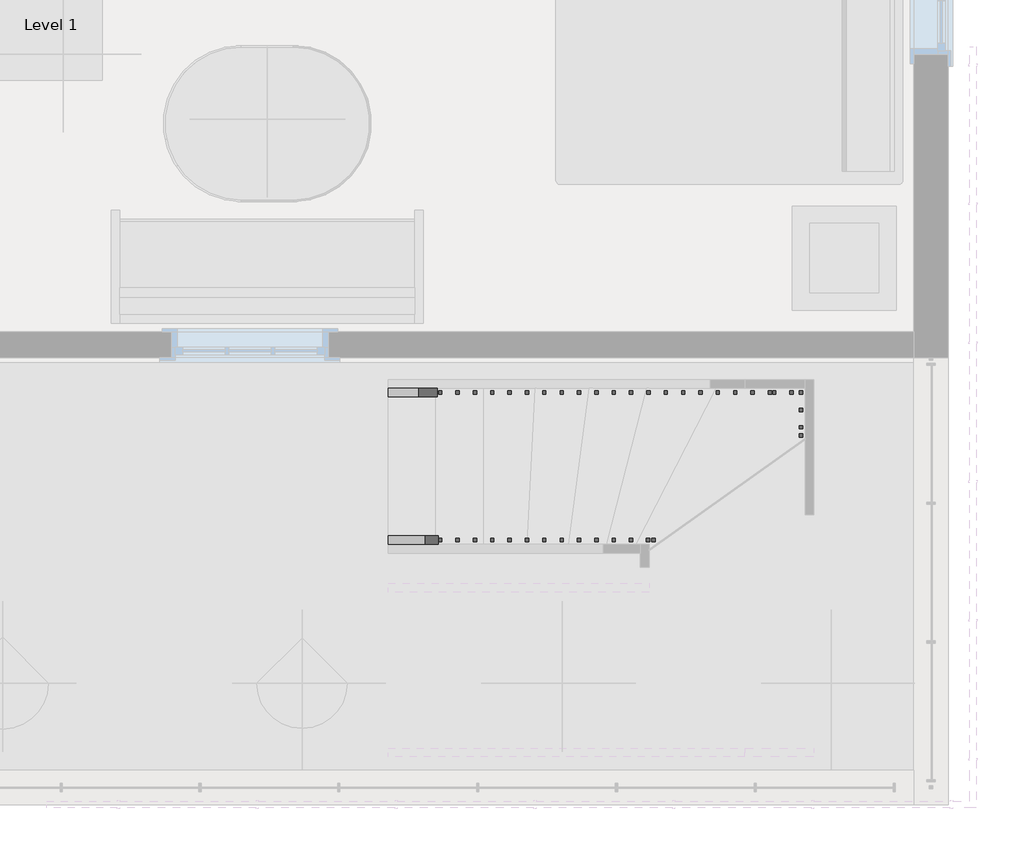
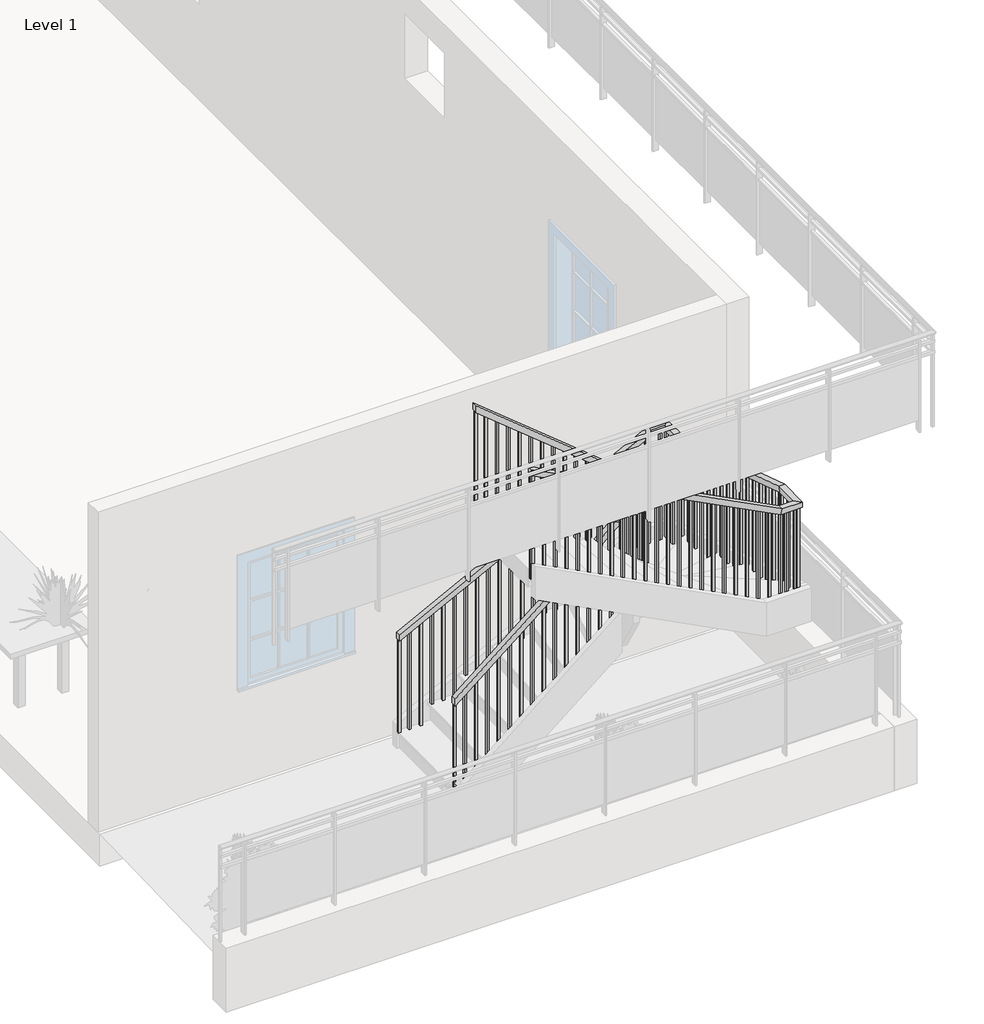
# One storey, part 2 of 5: 2 railings.
"""IFC4 building model written with IfcOpenShell, lengths in millimetres."""

from ifc_helpers import new_model, si_unit, frame, origin, place, context, project, spatial, polyline, outline, extrude, faceted_brep, element, save

model = new_model("IFC4")

# Units and contexts
model_context = context("Model", 3, world=origin())
ifc_project = project(units=[si_unit("LENGTHUNIT", "METRE", prefix="MILLI")], contexts=[model_context])

# Site, building, storey
site = spatial("IfcSite", under=ifc_project)
building = spatial("IfcBuilding", under=site)
storey = spatial("IfcBuildingStorey", under=building, Name="Level 1", Elevation=0.0)

# Railings
placement = place(None, origin())
element("IfcRailing", 1, ObjectType="Handrail - Rectangular", at=placement, inside=storey, context=model_context, shape_type="SolidModel", body=[
    faceted_brep([(-3203.9558053, -1061.3366944, 1025.2529681), (-3203.9558053, -1061.3366944, 959.7067088), (-3203.9558053, -1112.1366944, 959.7067088), (-3203.9558053, -1112.1366944, 1025.2529681), (-1752.4241134, -1061.3366944, 2208.7848338), (-1701.6241134, -1061.3366944, 2184.659247), (-1701.6241134, -1112.1366944, 2184.659247), (-1752.4241134, -1112.1366944, 2208.7848338), (-1752.4241134, -1061.3366944, 2414.6281882), (-1701.6241134, -1061.3366944, 2363.8281882), (-1701.6241134, -1112.1366944, 2363.8281882), (-1752.4241134, -1112.1366944, 2414.6281882), (-1625.4241134, -1061.3366944, 2414.6281882), (-1625.4241134, -1061.3366944, 2363.8281882), (-1676.2241134, -1112.1366944, 2363.8281882), (-1676.2241134, -1112.1366944, 2414.6281882), (-1625.4241134, -1188.3366944, 2414.6281882), (-1625.4241134, -1217.4580282, 2363.8281882), (-1676.2241134, -1217.4580282, 2363.8281882), (-1676.2241134, -1188.3366944, 2414.6281882), (-1625.4241134, -1315.3366944, 2631.5051451), (-1625.4241134, -1366.1366944, 2617.7256424), (-1676.2241134, -1366.1366944, 2617.7256424), (-1676.2241134, -1315.3366944, 2631.5051451), (-1625.4241134, -1315.3366944, 2837.3484995), (-1625.4241134, -1366.1366944, 2786.5484995), (-1676.2241134, -1366.1366944, 2786.5484995), (-1676.2241134, -1315.3366944, 2837.3484995), (-1625.4241134, -1442.3366944, 2837.3484995), (-1625.4241134, -1442.3366944, 2786.5484995), (-1676.2241134, -1391.5366944, 2786.5484995), (-1676.2241134, -1391.5366944, 2837.3484995), (-1752.4241134, -1442.3366944, 2837.3484995), (-1770.5095265, -1442.3366944, 2786.5484995), (-1770.5095265, -1391.5366944, 2786.5484995), (-1752.4241134, -1391.5366944, 2837.3484995), (-3203.9558053, -1442.3366944, 4020.8803652), (-3203.9558053, -1391.5366944, 4020.8803652), (-3203.9558053, -1391.5366944, 3955.3341059), (-3203.9558053, -1442.3366944, 3955.3341059)], [[[0, 1, 2, 3]], [[1, 0, 4, 5]], [[2, 1, 5, 6]], [[3, 2, 6, 7]], [[0, 3, 7, 4]], [[5, 4, 8, 9]], [[6, 5, 9, 10]], [[7, 6, 10, 11]], [[4, 7, 11, 8]], [[9, 8, 12, 13]], [[10, 9, 13, 14]], [[11, 10, 14, 15]], [[8, 11, 15, 12]], [[13, 12, 16, 17]], [[14, 13, 17, 18]], [[15, 14, 18, 19]], [[12, 15, 19, 16]], [[17, 16, 20, 21]], [[18, 17, 21, 22]], [[19, 18, 22, 23]], [[16, 19, 23, 20]], [[21, 20, 24, 25]], [[22, 21, 25, 26]], [[23, 22, 26, 27]], [[20, 23, 27, 24]], [[25, 24, 28, 29]], [[26, 25, 29, 30]], [[27, 26, 30, 31]], [[24, 27, 31, 28]], [[29, 28, 32, 33]], [[30, 29, 33, 34]], [[31, 30, 34, 35]], [[28, 31, 35, 32]], [[36, 37, 38, 39]], [[33, 32, 36, 39]], [[34, 33, 39, 38]], [[35, 34, 38, 37]], [[32, 35, 37, 36]]]),
    extrude(outline(polyline([(3866.2231262, -3094.6664698), (3881.7558784, -3113.7164698), (2878.6666667, -3113.7164698), (2878.6666667, -3094.6664698), (3866.2231262, -3094.6664698)])), frame((0.0, -1426.4616944, 0.0), z_axis=(0.0, 1.0, 0.0), x_axis=(0.0, 0.0, 1.0)), (0.0, 0.0, 1.0), 19.05),
    extrude(outline(polyline([(3783.3817813, -2993.0664698), (3798.9145334, -3012.1164698), (2878.6666667, -3012.1164698), (2878.6666667, -2993.0664698), (3783.3817813, -2993.0664698)])), frame((0.0, -1426.4616944, 0.0), z_axis=(0.0, 1.0, 0.0), x_axis=(0.0, 0.0, 1.0)), (0.0, 0.0, 1.0), 19.05),
    extrude(outline(polyline([(3700.5404364, -2891.4664698), (3716.0731885, -2910.5164698), (2709.3333333, -2910.5164698), (2709.3333333, -2891.4664698), (3700.5404364, -2891.4664698)])), frame((0.0, -1426.4616944, 0.0), z_axis=(0.0, 1.0, 0.0), x_axis=(0.0, 0.0, 1.0)), (0.0, 0.0, 1.0), 19.05),
    extrude(outline(polyline([(3617.6990914, -2789.8664698), (3633.2318436, -2808.9164698), (2709.3333333, -2808.9164698), (2709.3333333, -2789.8664698), (3617.6990914, -2789.8664698)])), frame((0.0, -1426.4616944, 0.0), z_axis=(0.0, 1.0, 0.0), x_axis=(0.0, 0.0, 1.0)), (0.0, 0.0, 1.0), 19.05),
    extrude(outline(polyline([(3534.8577465, -2688.2664698), (3550.3904987, -2707.3164698), (2709.3333333, -2707.3164698), (2709.3333333, -2688.2664698), (3534.8577465, -2688.2664698)])), frame((0.0, -1426.4616944, 0.0), z_axis=(0.0, 1.0, 0.0), x_axis=(0.0, 0.0, 1.0)), (0.0, 0.0, 1.0), 19.05),
    extrude(outline(polyline([(3452.0164016, -2586.6664698), (3467.5491538, -2605.7164698), (2540.0, -2605.7164698), (2540.0, -2586.6664698), (3452.0164016, -2586.6664698)])), frame((0.0, -1426.4616944, 0.0), z_axis=(0.0, 1.0, 0.0), x_axis=(0.0, 0.0, 1.0)), (0.0, 0.0, 1.0), 19.05),
    extrude(outline(polyline([(3369.1750567, -2485.0664698), (3384.7078088, -2504.1164698), (2540.0, -2504.1164698), (2540.0, -2485.0664698), (3369.1750567, -2485.0664698)])), frame((0.0, -1426.4616944, 0.0), z_axis=(0.0, 1.0, 0.0), x_axis=(0.0, 0.0, 1.0)), (0.0, 0.0, 1.0), 19.05),
    extrude(outline(polyline([(3286.3337117, -2383.4664698), (3301.8664639, -2402.5164698), (2540.0, -2402.5164698), (2540.0, -2383.4664698), (3286.3337117, -2383.4664698)])), frame((0.0, -1426.4616944, 0.0), z_axis=(0.0, 1.0, 0.0), x_axis=(0.0, 0.0, 1.0)), (0.0, 0.0, 1.0), 19.05),
    extrude(outline(polyline([(3203.4923668, -2281.8664698), (3219.025119, -2300.9164698), (2370.6666667, -2300.9164698), (2370.6666667, -2281.8664698), (3203.4923668, -2281.8664698)])), frame((0.0, -1426.4616944, 0.0), z_axis=(0.0, 1.0, 0.0), x_axis=(0.0, 0.0, 1.0)), (0.0, 0.0, 1.0), 19.05),
    extrude(outline(polyline([(3120.6510219, -2180.2664698), (3136.1837741, -2199.3164698), (2370.6666667, -2199.3164698), (2370.6666667, -2180.2664698), (3120.6510219, -2180.2664698)])), frame((0.0, -1426.4616944, 0.0), z_axis=(0.0, 1.0, 0.0), x_axis=(0.0, 0.0, 1.0)), (0.0, 0.0, 1.0), 19.05),
    extrude(outline(polyline([(3037.809677, -2078.6664698), (3053.3424291, -2097.7164698), (2201.3333333, -2097.7164698), (2201.3333333, -2078.6664698), (3037.809677, -2078.6664698)])), frame((0.0, -1426.4616944, 0.0), z_axis=(0.0, 1.0, 0.0), x_axis=(0.0, 0.0, 1.0)), (0.0, 0.0, 1.0), 19.05),
    extrude(outline(polyline([(2954.9683321, -1977.0664698), (2970.5010842, -1996.1164698), (2201.3333333, -1996.1164698), (2201.3333333, -1977.0664698), (2954.9683321, -1977.0664698)])), frame((0.0, -1426.4616944, 0.0), z_axis=(0.0, 1.0, 0.0), x_axis=(0.0, 0.0, 1.0)), (0.0, 0.0, 1.0), 19.05),
    extrude(outline(polyline([(2872.1269871, -1875.4664698), (2887.6597393, -1894.5164698), (2032.0, -1894.5164698), (2032.0, -1875.4664698), (2872.1269871, -1875.4664698)])), frame((0.0, -1426.4616944, 0.0), z_axis=(0.0, 1.0, 0.0), x_axis=(0.0, 0.0, 1.0)), (0.0, 0.0, 1.0), 19.05),
    extrude(outline(polyline([(2789.2856422, -1773.8664698), (2804.8183944, -1792.9164698), (2032.0, -1792.9164698), (2032.0, -1773.8664698), (2789.2856422, -1773.8664698)])), frame((0.0, -1426.4616944, 0.0), z_axis=(0.0, 1.0, 0.0), x_axis=(0.0, 0.0, 1.0)), (0.0, 0.0, 1.0), 19.05),
    extrude(outline(polyline([(-1314.2475981, 2529.115018), (-1295.1975981, 2496.5834745), (-1295.1975981, 1524.0), (-1314.2475981, 1524.0), (-1314.2475981, 2529.115018)])), frame((-1660.3491134, 0.0, 0.0), z_axis=(1.0, 0.0, 0.0), x_axis=(0.0, 1.0, 0.0)), (0.0, 0.0, 1.0), 19.05),
    extrude(outline(polyline([(-1212.6475981, 2355.6134525), (-1193.5975981, 2323.0819089), (-1193.5975981, 1524.0), (-1212.6475981, 1524.0), (-1212.6475981, 2355.6134525)])), frame((-1660.3491134, 0.0, 0.0), z_axis=(1.0, 0.0, 0.0), x_axis=(0.0, 1.0, 0.0)), (0.0, 0.0, 1.0), 19.05),
    extrude(outline(polyline([(2127.2519138, -1772.0308053), (2111.7191617, -1791.0808053), (1016.0, -1791.0808053), (1016.0, -1772.0308053), (2127.2519138, -1772.0308053)])), frame((0.0, -1096.2616944, 0.0), z_axis=(0.0, 1.0, 0.0), x_axis=(0.0, 0.0, 1.0)), (0.0, 0.0, 1.0), 19.05),
    extrude(outline(polyline([(2044.4105689, -1873.6308053), (2028.8778167, -1892.6808053), (1016.0, -1892.6808053), (1016.0, -1873.6308053), (2044.4105689, -1873.6308053)])), frame((0.0, -1096.2616944, 0.0), z_axis=(0.0, 1.0, 0.0), x_axis=(0.0, 0.0, 1.0)), (0.0, 0.0, 1.0), 19.05),
    extrude(outline(polyline([(1961.569224, -1975.2308053), (1946.0364718, -1994.2808053), (846.6666667, -1994.2808053), (846.6666667, -1975.2308053), (1961.569224, -1975.2308053)])), frame((0.0, -1096.2616944, 0.0), z_axis=(0.0, 1.0, 0.0), x_axis=(0.0, 0.0, 1.0)), (0.0, 0.0, 1.0), 19.05),
    extrude(outline(polyline([(1878.7278791, -2076.8308053), (1863.1951269, -2095.8808053), (846.6666667, -2095.8808053), (846.6666667, -2076.8308053), (1878.7278791, -2076.8308053)])), frame((0.0, -1096.2616944, 0.0), z_axis=(0.0, 1.0, 0.0), x_axis=(0.0, 0.0, 1.0)), (0.0, 0.0, 1.0), 19.05),
    extrude(outline(polyline([(1795.8865341, -2178.4308053), (1780.353782, -2197.4808053), (677.3333333, -2197.4808053), (677.3333333, -2178.4308053), (1795.8865341, -2178.4308053)])), frame((0.0, -1096.2616944, 0.0), z_axis=(0.0, 1.0, 0.0), x_axis=(0.0, 0.0, 1.0)), (0.0, 0.0, 1.0), 19.05),
    extrude(outline(polyline([(1713.0451892, -2280.0308053), (1697.5124371, -2299.0808053), (677.3333333, -2299.0808053), (677.3333333, -2280.0308053), (1713.0451892, -2280.0308053)])), frame((0.0, -1096.2616944, 0.0), z_axis=(0.0, 1.0, 0.0), x_axis=(0.0, 0.0, 1.0)), (0.0, 0.0, 1.0), 19.05),
    extrude(outline(polyline([(1630.2038443, -2381.6308053), (1614.6710921, -2400.6808053), (508.0, -2400.6808053), (508.0, -2381.6308053), (1630.2038443, -2381.6308053)])), frame((0.0, -1096.2616944, 0.0), z_axis=(0.0, 1.0, 0.0), x_axis=(0.0, 0.0, 1.0)), (0.0, 0.0, 1.0), 19.05),
    extrude(outline(polyline([(1547.3624994, -2483.2308053), (1531.8297472, -2502.2808053), (508.0, -2502.2808053), (508.0, -2483.2308053), (1547.3624994, -2483.2308053)])), frame((0.0, -1096.2616944, 0.0), z_axis=(0.0, 1.0, 0.0), x_axis=(0.0, 0.0, 1.0)), (0.0, 0.0, 1.0), 19.05),
    extrude(outline(polyline([(1464.5211545, -2584.8308053), (1448.9884023, -2603.8808053), (508.0, -2603.8808053), (508.0, -2584.8308053), (1464.5211545, -2584.8308053)])), frame((0.0, -1096.2616944, 0.0), z_axis=(0.0, 1.0, 0.0), x_axis=(0.0, 0.0, 1.0)), (0.0, 0.0, 1.0), 19.05),
    extrude(outline(polyline([(1381.6798095, -2686.4308053), (1366.1470574, -2705.4808053), (338.6666667, -2705.4808053), (338.6666667, -2686.4308053), (1381.6798095, -2686.4308053)])), frame((0.0, -1096.2616944, 0.0), z_axis=(0.0, 1.0, 0.0), x_axis=(0.0, 0.0, 1.0)), (0.0, 0.0, 1.0), 19.05),
    extrude(outline(polyline([(1298.8384646, -2788.0308053), (1283.3057124, -2807.0808053), (338.6666667, -2807.0808053), (338.6666667, -2788.0308053), (1298.8384646, -2788.0308053)])), frame((0.0, -1096.2616944, 0.0), z_axis=(0.0, 1.0, 0.0), x_axis=(0.0, 0.0, 1.0)), (0.0, 0.0, 1.0), 19.05),
    extrude(outline(polyline([(1215.9971197, -2889.6308053), (1200.4643675, -2908.6808053), (338.6666667, -2908.6808053), (338.6666667, -2889.6308053), (1215.9971197, -2889.6308053)])), frame((0.0, -1096.2616944, 0.0), z_axis=(0.0, 1.0, 0.0), x_axis=(0.0, 0.0, 1.0)), (0.0, 0.0, 1.0), 19.05),
    extrude(outline(polyline([(1133.1557748, -2991.2308053), (1117.6230226, -3010.2808053), (169.3333333, -3010.2808053), (169.3333333, -2991.2308053), (1133.1557748, -2991.2308053)])), frame((0.0, -1096.2616944, 0.0), z_axis=(0.0, 1.0, 0.0), x_axis=(0.0, 0.0, 1.0)), (0.0, 0.0, 1.0), 19.05),
    extrude(outline(polyline([(1050.3144298, -3092.8308053), (1034.7816777, -3111.8808053), (169.3333333, -3111.8808053), (169.3333333, -3092.8308053), (1050.3144298, -3092.8308053)])), frame((0.0, -1096.2616944, 0.0), z_axis=(0.0, 1.0, 0.0), x_axis=(0.0, 0.0, 1.0)), (0.0, 0.0, 1.0), 19.05),
    extrude(outline(polyline([(-1672.2664698, -1407.4116944), (-1672.2664698, -1426.4616944), (-1691.3164698, -1426.4616944), (-1691.3164698, -1407.4116944), (-1672.2664698, -1407.4116944)])), frame((0.0, 0.0, 1862.6666667), z_axis=(0.0, 0.0, 1.0), x_axis=(1.0, 0.0, 0.0)), (0.0, 0.0, 1.0), 923.8818329),
    extrude(outline(polyline([(-1660.3491134, -1407.4116944), (-1641.2991134, -1407.4116944), (-1641.2991134, -1426.4616944), (-1660.3491134, -1426.4616944), (-1660.3491134, -1407.4116944)])), frame((0.0, 0.0, 1862.6666667), z_axis=(0.0, 0.0, 1.0), x_axis=(1.0, 0.0, 0.0)), (0.0, 0.0, 1.0), 923.8818329),
    extrude(outline(polyline([(-1660.3491134, -1392.6257906), (-1641.2991134, -1392.6257906), (-1641.2991134, -1411.6757906), (-1660.3491134, -1411.6757906), (-1660.3491134, -1392.6257906)])), frame((0.0, 0.0, 1693.3333333), z_axis=(0.0, 0.0, 1.0), x_axis=(1.0, 0.0, 0.0)), (0.0, 0.0, 1.0), 1093.2151662),
    extrude(outline(polyline([(-1660.3491134, -1091.9975981), (-1641.2991134, -1091.9975981), (-1641.2991134, -1111.0475981), (-1660.3491134, -1111.0475981), (-1660.3491134, -1091.9975981)])), frame((0.0, 0.0, 1354.6666667), z_axis=(0.0, 0.0, 1.0), x_axis=(1.0, 0.0, 0.0)), (0.0, 0.0, 1.0), 1009.1615215),
    extrude(outline(polyline([(-1660.3491134, -1096.2616944), (-1660.3491134, -1077.2116944), (-1641.2991134, -1077.2116944), (-1641.2991134, -1096.2616944), (-1660.3491134, -1096.2616944)])), frame((0.0, 0.0, 1185.3333333), z_axis=(0.0, 0.0, 1.0), x_axis=(1.0, 0.0, 0.0)), (0.0, 0.0, 1.0), 1178.4948549),
    extrude(outline(polyline([(-1691.3164698, -1096.2616944), (-1691.3164698, -1077.2116944), (-1672.2664698, -1077.2116944), (-1672.2664698, -1096.2616944), (-1691.3164698, -1096.2616944)])), frame((0.0, 0.0, 1185.3333333), z_axis=(0.0, 0.0, 1.0), x_axis=(1.0, 0.0, 0.0)), (0.0, 0.0, 1.0), 1178.4948549),
    extrude(outline(polyline([(3939.8013537, -3184.9058053), (3955.3341059, -3203.9558053), (2878.6666667, -3203.9558053), (2878.6666667, -3184.9058053), (3939.8013537, -3184.9058053)])), frame((0.0, -1426.4616944, 0.0), z_axis=(0.0, 1.0, 0.0), x_axis=(0.0, 0.0, 1.0)), (0.0, 0.0, 1.0), 19.05),
    extrude(outline(polyline([(975.239461, -3184.9058053), (959.7067088, -3203.9558053), (169.3333333, -3203.9558053), (169.3333333, -3184.9058053), (975.239461, -3184.9058053)])), frame((0.0, -1096.2616944, 0.0), z_axis=(0.0, 1.0, 0.0), x_axis=(0.0, 0.0, 1.0)), (0.0, 0.0, 1.0), 19.05),
])
element("IfcRailing", 2, ObjectType="Handrail - Rectangular", at=placement, inside=storey, context=model_context, shape_type="SolidModel", body=[
    faceted_brep([(-3203.9558053, -197.7366944, 1109.0771751), (-3203.9558053, -197.7366944, 1051.9280057), (-3203.9558053, -248.5366944, 1051.9280057), (-3203.9558053, -248.5366944, 1109.0771751), (-943.9739488, -197.7366944, 2273.7644996), (-931.6538975, -197.7366944, 2222.9644996), (-931.6538975, -248.5366944, 2222.9644996), (-943.9739488, -248.5366944, 2273.7644996), (-761.8241134, -197.7366944, 2273.7644996), (-761.8241134, -197.7366944, 2222.9644996), (-812.6241134, -248.5366944, 2222.9644996), (-812.6241134, -248.5366944, 2273.7644996), (-761.8241134, -474.890647, 2273.7644996), (-761.8241134, -482.8412231, 2222.9644996), (-812.6241134, -482.8412231, 2222.9644996), (-812.6241134, -474.890647, 2273.7644996), (-761.8241134, -2028.7827418, 2772.3688337), (-761.8241134, -2036.7333179, 2721.5688337), (-812.6241134, -2036.7333179, 2721.5688337), (-812.6241134, -2028.7827418, 2772.3688337), (-761.8241134, -2305.9366944, 2772.3688337), (-761.8241134, -2305.9366944, 2721.5688337), (-812.6241134, -2255.1366944, 2721.5688337), (-812.6241134, -2255.1366944, 2772.3688337), (-943.9739488, -2305.9366944, 2772.3688337), (-956.2940001, -2305.9366944, 2721.5688337), (-956.2940001, -2255.1366944, 2721.5688337), (-943.9739488, -2255.1366944, 2772.3688337), (-3203.9558053, -2305.9366944, 3937.0561582), (-3203.9558053, -2255.1366944, 3937.0561582), (-3203.9558053, -2255.1366944, 3879.9069889), (-3203.9558053, -2305.9366944, 3879.9069889)], [[[0, 1, 2, 3]], [[1, 0, 4, 5]], [[2, 1, 5, 6]], [[3, 2, 6, 7]], [[0, 3, 7, 4]], [[5, 4, 8, 9]], [[6, 5, 9, 10]], [[7, 6, 10, 11]], [[4, 7, 11, 8]], [[9, 8, 12, 13]], [[10, 9, 13, 14]], [[11, 10, 14, 15]], [[8, 11, 15, 12]], [[13, 12, 16, 17]], [[14, 13, 17, 18]], [[15, 14, 18, 19]], [[12, 15, 19, 16]], [[17, 16, 20, 21]], [[18, 17, 21, 22]], [[19, 18, 22, 23]], [[16, 19, 23, 20]], [[21, 20, 24, 25]], [[22, 21, 25, 26]], [[23, 22, 26, 27]], [[20, 23, 27, 24]], [[28, 29, 30, 31]], [[25, 24, 28, 31]], [[26, 25, 31, 30]], [[27, 26, 30, 29]], [[24, 27, 29, 28]]]),
    extrude(outline(polyline([(3872.0443296, -3188.6989488), (2878.6666667, -3188.6989488), (2878.6666667, -3169.6489488), (3862.2268642, -3169.6489488), (3872.0443296, -3188.6989488)])), frame((0.0, -2290.0616944, 0.0), z_axis=(0.0, 1.0, 0.0), x_axis=(0.0, 0.0, 1.0)), (0.0, 0.0, 1.0), 19.05),
    extrude(outline(polyline([(3819.6845145, -3087.0989488), (2878.6666667, -3087.0989488), (2878.6666667, -3068.0489488), (3809.8670491, -3068.0489488), (3819.6845145, -3087.0989488)])), frame((0.0, -2290.0616944, 0.0), z_axis=(0.0, 1.0, 0.0), x_axis=(0.0, 0.0, 1.0)), (0.0, 0.0, 1.0), 19.05),
    extrude(outline(polyline([(3767.3246993, -2985.4989488), (2878.6666667, -2985.4989488), (2878.6666667, -2966.4489488), (3757.507234, -2966.4489488), (3767.3246993, -2985.4989488)])), frame((0.0, -2290.0616944, 0.0), z_axis=(0.0, 1.0, 0.0), x_axis=(0.0, 0.0, 1.0)), (0.0, 0.0, 1.0), 19.05),
    extrude(outline(polyline([(3714.9648842, -2883.8989488), (2709.3333333, -2883.8989488), (2709.3333333, -2864.8489488), (3705.1474189, -2864.8489488), (3714.9648842, -2883.8989488)])), frame((0.0, -2290.0616944, 0.0), z_axis=(0.0, 1.0, 0.0), x_axis=(0.0, 0.0, 1.0)), (0.0, 0.0, 1.0), 19.05),
    extrude(outline(polyline([(3662.6050691, -2782.2989488), (2709.3333333, -2782.2989488), (2709.3333333, -2763.2489488), (3652.7876038, -2763.2489488), (3662.6050691, -2782.2989488)])), frame((0.0, -2290.0616944, 0.0), z_axis=(0.0, 1.0, 0.0), x_axis=(0.0, 0.0, 1.0)), (0.0, 0.0, 1.0), 19.05),
    extrude(outline(polyline([(3610.245254, -2680.6989488), (2709.3333333, -2680.6989488), (2709.3333333, -2661.6489488), (3600.4277887, -2661.6489488), (3610.245254, -2680.6989488)])), frame((0.0, -2290.0616944, 0.0), z_axis=(0.0, 1.0, 0.0), x_axis=(0.0, 0.0, 1.0)), (0.0, 0.0, 1.0), 19.05),
    extrude(outline(polyline([(3557.8854389, -2579.0989488), (2540.0, -2579.0989488), (2540.0, -2560.0489488), (3548.0679735, -2560.0489488), (3557.8854389, -2579.0989488)])), frame((0.0, -2290.0616944, 0.0), z_axis=(0.0, 1.0, 0.0), x_axis=(0.0, 0.0, 1.0)), (0.0, 0.0, 1.0), 19.05),
    extrude(outline(polyline([(3505.5256238, -2477.4989488), (2540.0, -2477.4989488), (2540.0, -2458.4489488), (3495.7081584, -2458.4489488), (3505.5256238, -2477.4989488)])), frame((0.0, -2290.0616944, 0.0), z_axis=(0.0, 1.0, 0.0), x_axis=(0.0, 0.0, 1.0)), (0.0, 0.0, 1.0), 19.05),
    extrude(outline(polyline([(3453.1658086, -2375.8989488), (2540.0, -2375.8989488), (2540.0, -2356.8489488), (3443.3483433, -2356.8489488), (3453.1658086, -2375.8989488)])), frame((0.0, -2290.0616944, 0.0), z_axis=(0.0, 1.0, 0.0), x_axis=(0.0, 0.0, 1.0)), (0.0, 0.0, 1.0), 19.05),
    extrude(outline(polyline([(3400.8059935, -2274.2989488), (2370.6666667, -2274.2989488), (2370.6666667, -2255.2489488), (3390.9885282, -2255.2489488), (3400.8059935, -2274.2989488)])), frame((0.0, -2290.0616944, 0.0), z_axis=(0.0, 1.0, 0.0), x_axis=(0.0, 0.0, 1.0)), (0.0, 0.0, 1.0), 19.05),
    extrude(outline(polyline([(3348.4461784, -2172.6989488), (2370.6666667, -2172.6989488), (2370.6666667, -2153.6489488), (3338.6287131, -2153.6489488), (3348.4461784, -2172.6989488)])), frame((0.0, -2290.0616944, 0.0), z_axis=(0.0, 1.0, 0.0), x_axis=(0.0, 0.0, 1.0)), (0.0, 0.0, 1.0), 19.05),
    extrude(outline(polyline([(3296.0863633, -2071.0989488), (2370.6666667, -2071.0989488), (2370.6666667, -2052.0489488), (3286.268898, -2052.0489488), (3296.0863633, -2071.0989488)])), frame((0.0, -2290.0616944, 0.0), z_axis=(0.0, 1.0, 0.0), x_axis=(0.0, 0.0, 1.0)), (0.0, 0.0, 1.0), 19.05),
    extrude(outline(polyline([(3243.7265482, -1969.4989488), (2201.3333333, -1969.4989488), (2201.3333333, -1950.4489488), (3233.9090828, -1950.4489488), (3243.7265482, -1969.4989488)])), frame((0.0, -2290.0616944, 0.0), z_axis=(0.0, 1.0, 0.0), x_axis=(0.0, 0.0, 1.0)), (0.0, 0.0, 1.0), 19.05),
    extrude(outline(polyline([(3191.3667331, -1867.8989488), (2201.3333333, -1867.8989488), (2201.3333333, -1848.8489488), (3181.5492677, -1848.8489488), (3191.3667331, -1867.8989488)])), frame((0.0, -2290.0616944, 0.0), z_axis=(0.0, 1.0, 0.0), x_axis=(0.0, 0.0, 1.0)), (0.0, 0.0, 1.0), 19.05),
    extrude(outline(polyline([(3139.0069179, -1766.2989488), (2201.3333333, -1766.2989488), (2201.3333333, -1747.2489488), (3129.1894526, -1747.2489488), (3139.0069179, -1766.2989488)])), frame((0.0, -2290.0616944, 0.0), z_axis=(0.0, 1.0, 0.0), x_axis=(0.0, 0.0, 1.0)), (0.0, 0.0, 1.0), 19.05),
    extrude(outline(polyline([(3086.6471028, -1664.6989488), (2032.0, -1664.6989488), (2032.0, -1645.6489488), (3076.8296375, -1645.6489488), (3086.6471028, -1664.6989488)])), frame((0.0, -2290.0616944, 0.0), z_axis=(0.0, 1.0, 0.0), x_axis=(0.0, 0.0, 1.0)), (0.0, 0.0, 1.0), 19.05),
    extrude(outline(polyline([(3034.2872877, -1563.0989488), (2032.0, -1563.0989488), (2032.0, -1544.0489488), (3024.4698224, -1544.0489488), (3034.2872877, -1563.0989488)])), frame((0.0, -2290.0616944, 0.0), z_axis=(0.0, 1.0, 0.0), x_axis=(0.0, 0.0, 1.0)), (0.0, 0.0, 1.0), 19.05),
    extrude(outline(polyline([(2981.9274726, -1461.4989488), (2032.0, -1461.4989488), (2032.0, -1442.4489488), (2972.1100073, -1442.4489488), (2981.9274726, -1461.4989488)])), frame((0.0, -2290.0616944, 0.0), z_axis=(0.0, 1.0, 0.0), x_axis=(0.0, 0.0, 1.0)), (0.0, 0.0, 1.0), 19.05),
    extrude(outline(polyline([(2929.5676575, -1359.8989488), (2032.0, -1359.8989488), (2032.0, -1340.8489488), (2919.7501921, -1340.8489488), (2929.5676575, -1359.8989488)])), frame((0.0, -2290.0616944, 0.0), z_axis=(0.0, 1.0, 0.0), x_axis=(0.0, 0.0, 1.0)), (0.0, 0.0, 1.0), 19.05),
    extrude(outline(polyline([(2877.2078424, -1258.2989488), (1862.6666667, -1258.2989488), (1862.6666667, -1239.2489488), (2867.390377, -1239.2489488), (2877.2078424, -1258.2989488)])), frame((0.0, -2290.0616944, 0.0), z_axis=(0.0, 1.0, 0.0), x_axis=(0.0, 0.0, 1.0)), (0.0, 0.0, 1.0), 19.05),
    extrude(outline(polyline([(2824.8480272, -1156.6989488), (1862.6666667, -1156.6989488), (1862.6666667, -1137.6489488), (2815.0305619, -1137.6489488), (2824.8480272, -1156.6989488)])), frame((0.0, -2290.0616944, 0.0), z_axis=(0.0, 1.0, 0.0), x_axis=(0.0, 0.0, 1.0)), (0.0, 0.0, 1.0), 19.05),
    extrude(outline(polyline([(2772.4882121, -1055.0989488), (1862.6666667, -1055.0989488), (1862.6666667, -1036.0489488), (2762.6707468, -1036.0489488), (2772.4882121, -1055.0989488)])), frame((0.0, -2290.0616944, 0.0), z_axis=(0.0, 1.0, 0.0), x_axis=(0.0, 0.0, 1.0)), (0.0, 0.0, 1.0), 19.05),
    extrude(outline(polyline([(-879.2991134, -2290.0616944), (-898.3491134, -2290.0616944), (-898.3491134, -2271.0116944), (-879.2991134, -2271.0116944), (-879.2991134, -2290.0616944)])), frame((0.0, 0.0, 1862.6666667), z_axis=(0.0, 0.0, 1.0), x_axis=(1.0, 0.0, 0.0)), (0.0, 0.0, 1.0), 858.902167),
    extrude(outline(polyline([(-777.6991134, -2222.4577418), (-777.6991134, -2241.5077418), (-796.7491134, -2241.5077418), (-796.7491134, -2222.4577418), (-777.6991134, -2222.4577418)])), frame((0.0, 0.0, 1862.6666667), z_axis=(0.0, 0.0, 1.0), x_axis=(1.0, 0.0, 0.0)), (0.0, 0.0, 1.0), 858.902167),
    extrude(outline(polyline([(-777.6991134, -2120.8577418), (-777.6991134, -2139.9077418), (-796.7491134, -2139.9077418), (-796.7491134, -2120.8577418), (-777.6991134, -2120.8577418)])), frame((0.0, 0.0, 1862.6666667), z_axis=(0.0, 0.0, 1.0), x_axis=(1.0, 0.0, 0.0)), (0.0, 0.0, 1.0), 858.902167),
    extrude(outline(polyline([(-1989.365647, 2706.3697564), (-1989.365647, 1693.3333333), (-2008.415647, 1693.3333333), (-2008.415647, 2712.4824155), (-1989.365647, 2706.3697564)])), frame((-796.7491134, 0.0, 0.0), z_axis=(1.0, 0.0, 0.0), x_axis=(0.0, 1.0, 0.0)), (0.0, 0.0, 1.0), 19.05),
    extrude(outline(polyline([(-1887.765647, 2673.7689082), (-1887.765647, 1693.3333333), (-1906.815647, 1693.3333333), (-1906.815647, 2679.8815673), (-1887.765647, 2673.7689082)])), frame((-796.7491134, 0.0, 0.0), z_axis=(1.0, 0.0, 0.0), x_axis=(0.0, 1.0, 0.0)), (0.0, 0.0, 1.0), 19.05),
    extrude(outline(polyline([(-1786.165647, 2641.16806), (-1786.165647, 1693.3333333), (-1805.215647, 1693.3333333), (-1805.215647, 2647.280719), (-1786.165647, 2641.16806)])), frame((-796.7491134, 0.0, 0.0), z_axis=(1.0, 0.0, 0.0), x_axis=(0.0, 1.0, 0.0)), (0.0, 0.0, 1.0), 19.05),
    extrude(outline(polyline([(-1684.565647, 2608.5672118), (-1684.565647, 1693.3333333), (-1703.615647, 1693.3333333), (-1703.615647, 2614.6798708), (-1684.565647, 2608.5672118)])), frame((-796.7491134, 0.0, 0.0), z_axis=(1.0, 0.0, 0.0), x_axis=(0.0, 1.0, 0.0)), (0.0, 0.0, 1.0), 19.05),
    extrude(outline(polyline([(-1582.965647, 2575.9663635), (-1582.965647, 1693.3333333), (-1602.015647, 1693.3333333), (-1602.015647, 2582.0790226), (-1582.965647, 2575.9663635)])), frame((-796.7491134, 0.0, 0.0), z_axis=(1.0, 0.0, 0.0), x_axis=(0.0, 1.0, 0.0)), (0.0, 0.0, 1.0), 19.05),
    extrude(outline(polyline([(-1481.365647, 2543.3655153), (-1481.365647, 1693.3333333), (-1500.415647, 1693.3333333), (-1500.415647, 2549.4781744), (-1481.365647, 2543.3655153)])), frame((-796.7491134, 0.0, 0.0), z_axis=(1.0, 0.0, 0.0), x_axis=(0.0, 1.0, 0.0)), (0.0, 0.0, 1.0), 19.05),
    extrude(outline(polyline([(-1379.765647, 2510.7646671), (-1379.765647, 1524.0), (-1398.815647, 1524.0), (-1398.815647, 2516.8773261), (-1379.765647, 2510.7646671)])), frame((-796.7491134, 0.0, 0.0), z_axis=(1.0, 0.0, 0.0), x_axis=(0.0, 1.0, 0.0)), (0.0, 0.0, 1.0), 19.05),
    extrude(outline(polyline([(-1278.165647, 2478.1638189), (-1278.165647, 1524.0), (-1297.215647, 1524.0), (-1297.215647, 2484.2764779), (-1278.165647, 2478.1638189)])), frame((-796.7491134, 0.0, 0.0), z_axis=(1.0, 0.0, 0.0), x_axis=(0.0, 1.0, 0.0)), (0.0, 0.0, 1.0), 19.05),
    extrude(outline(polyline([(-1176.565647, 2445.5629706), (-1176.565647, 1524.0), (-1195.615647, 1524.0), (-1195.615647, 2451.6756297), (-1176.565647, 2445.5629706)])), frame((-796.7491134, 0.0, 0.0), z_axis=(1.0, 0.0, 0.0), x_axis=(0.0, 1.0, 0.0)), (0.0, 0.0, 1.0), 19.05),
    extrude(outline(polyline([(-1074.965647, 2412.9621224), (-1074.965647, 1524.0), (-1094.015647, 1524.0), (-1094.015647, 2419.0747814), (-1074.965647, 2412.9621224)])), frame((-796.7491134, 0.0, 0.0), z_axis=(1.0, 0.0, 0.0), x_axis=(0.0, 1.0, 0.0)), (0.0, 0.0, 1.0), 19.05),
    extrude(outline(polyline([(-973.365647, 2380.3612742), (-973.365647, 1354.6666667), (-992.415647, 1354.6666667), (-992.415647, 2386.4739332), (-973.365647, 2380.3612742)])), frame((-796.7491134, 0.0, 0.0), z_axis=(1.0, 0.0, 0.0), x_axis=(0.0, 1.0, 0.0)), (0.0, 0.0, 1.0), 19.05),
    extrude(outline(polyline([(-871.765647, 2347.7604259), (-871.765647, 1354.6666667), (-890.815647, 1354.6666667), (-890.815647, 2353.873085), (-871.765647, 2347.7604259)])), frame((-796.7491134, 0.0, 0.0), z_axis=(1.0, 0.0, 0.0), x_axis=(0.0, 1.0, 0.0)), (0.0, 0.0, 1.0), 19.05),
    extrude(outline(polyline([(-770.165647, 2315.1595777), (-770.165647, 1354.6666667), (-789.215647, 1354.6666667), (-789.215647, 2321.2722368), (-770.165647, 2315.1595777)])), frame((-796.7491134, 0.0, 0.0), z_axis=(1.0, 0.0, 0.0), x_axis=(0.0, 1.0, 0.0)), (0.0, 0.0, 1.0), 19.05),
    extrude(outline(polyline([(-668.565647, 2282.5587295), (-668.565647, 1354.6666667), (-687.615647, 1354.6666667), (-687.615647, 2288.6713885), (-668.565647, 2282.5587295)])), frame((-796.7491134, 0.0, 0.0), z_axis=(1.0, 0.0, 0.0), x_axis=(0.0, 1.0, 0.0)), (0.0, 0.0, 1.0), 19.05),
    extrude(outline(polyline([(-566.965647, 2249.9578813), (-566.965647, 1354.6666667), (-586.015647, 1354.6666667), (-586.015647, 2256.0705403), (-566.965647, 2249.9578813)])), frame((-796.7491134, 0.0, 0.0), z_axis=(1.0, 0.0, 0.0), x_axis=(0.0, 1.0, 0.0)), (0.0, 0.0, 1.0), 19.05),
    extrude(outline(polyline([(-777.6991134, -416.8116944), (-777.6991134, -435.8616944), (-796.7491134, -435.8616944), (-796.7491134, -416.8116944), (-777.6991134, -416.8116944)])), frame((0.0, 0.0, 1185.3333333), z_axis=(0.0, 0.0, 1.0), x_axis=(1.0, 0.0, 0.0)), (0.0, 0.0, 1.0), 1037.6311663),
    extrude(outline(polyline([(-777.6991134, -315.2116944), (-777.6991134, -334.2616944), (-796.7491134, -334.2616944), (-796.7491134, -315.2116944), (-777.6991134, -315.2116944)])), frame((0.0, 0.0, 1185.3333333), z_axis=(0.0, 0.0, 1.0), x_axis=(1.0, 0.0, 0.0)), (0.0, 0.0, 1.0), 1037.6311663),
    extrude(outline(polyline([(-851.8989488, -213.6116944), (-832.8489488, -213.6116944), (-832.8489488, -232.6616944), (-851.8989488, -232.6616944), (-851.8989488, -213.6116944)])), frame((0.0, 0.0, 1185.3333333), z_axis=(0.0, 0.0, 1.0), x_axis=(1.0, 0.0, 0.0)), (0.0, 0.0, 1.0), 1037.6311663),
    extrude(outline(polyline([(2198.9352056, -978.2808053), (1185.3333333, -978.2808053), (1185.3333333, -959.2308053), (2208.752671, -959.2308053), (2198.9352056, -978.2808053)])), frame((0.0, -232.6616944, 0.0), z_axis=(0.0, 1.0, 0.0), x_axis=(0.0, 0.0, 1.0)), (0.0, 0.0, 1.0), 19.05),
    extrude(outline(polyline([(2146.5753905, -1079.8808053), (1185.3333333, -1079.8808053), (1185.3333333, -1060.8308053), (2156.3928558, -1060.8308053), (2146.5753905, -1079.8808053)])), frame((0.0, -232.6616944, 0.0), z_axis=(0.0, 1.0, 0.0), x_axis=(0.0, 0.0, 1.0)), (0.0, 0.0, 1.0), 19.05),
    extrude(outline(polyline([(2094.2155754, -1181.4808053), (1185.3333333, -1181.4808053), (1185.3333333, -1162.4308053), (2104.0330407, -1162.4308053), (2094.2155754, -1181.4808053)])), frame((0.0, -232.6616944, 0.0), z_axis=(0.0, 1.0, 0.0), x_axis=(0.0, 0.0, 1.0)), (0.0, 0.0, 1.0), 19.05),
    extrude(outline(polyline([(2041.8557603, -1283.0808053), (1185.3333333, -1283.0808053), (1185.3333333, -1264.0308053), (2051.6732256, -1264.0308053), (2041.8557603, -1283.0808053)])), frame((0.0, -232.6616944, 0.0), z_axis=(0.0, 1.0, 0.0), x_axis=(0.0, 0.0, 1.0)), (0.0, 0.0, 1.0), 19.05),
    extrude(outline(polyline([(1989.4959452, -1384.6808053), (1016.0, -1384.6808053), (1016.0, -1365.6308053), (1999.3134105, -1365.6308053), (1989.4959452, -1384.6808053)])), frame((0.0, -232.6616944, 0.0), z_axis=(0.0, 1.0, 0.0), x_axis=(0.0, 0.0, 1.0)), (0.0, 0.0, 1.0), 19.05),
    extrude(outline(polyline([(1937.13613, -1486.2808053), (1016.0, -1486.2808053), (1016.0, -1467.2308053), (1946.9535954, -1467.2308053), (1937.13613, -1486.2808053)])), frame((0.0, -232.6616944, 0.0), z_axis=(0.0, 1.0, 0.0), x_axis=(0.0, 0.0, 1.0)), (0.0, 0.0, 1.0), 19.05),
    extrude(outline(polyline([(1884.7763149, -1587.8808053), (1016.0, -1587.8808053), (1016.0, -1568.8308053), (1894.5937803, -1568.8308053), (1884.7763149, -1587.8808053)])), frame((0.0, -232.6616944, 0.0), z_axis=(0.0, 1.0, 0.0), x_axis=(0.0, 0.0, 1.0)), (0.0, 0.0, 1.0), 19.05),
    extrude(outline(polyline([(1832.4164998, -1689.4808053), (1016.0, -1689.4808053), (1016.0, -1670.4308053), (1842.2339651, -1670.4308053), (1832.4164998, -1689.4808053)])), frame((0.0, -232.6616944, 0.0), z_axis=(0.0, 1.0, 0.0), x_axis=(0.0, 0.0, 1.0)), (0.0, 0.0, 1.0), 19.05),
    extrude(outline(polyline([(1780.0566847, -1791.0808053), (846.6666667, -1791.0808053), (846.6666667, -1772.0308053), (1789.87415, -1772.0308053), (1780.0566847, -1791.0808053)])), frame((0.0, -232.6616944, 0.0), z_axis=(0.0, 1.0, 0.0), x_axis=(0.0, 0.0, 1.0)), (0.0, 0.0, 1.0), 19.05),
    extrude(outline(polyline([(1727.6968696, -1892.6808053), (846.6666667, -1892.6808053), (846.6666667, -1873.6308053), (1737.5143349, -1873.6308053), (1727.6968696, -1892.6808053)])), frame((0.0, -232.6616944, 0.0), z_axis=(0.0, 1.0, 0.0), x_axis=(0.0, 0.0, 1.0)), (0.0, 0.0, 1.0), 19.05),
    extrude(outline(polyline([(1675.3370545, -1994.2808053), (846.6666667, -1994.2808053), (846.6666667, -1975.2308053), (1685.1545198, -1975.2308053), (1675.3370545, -1994.2808053)])), frame((0.0, -232.6616944, 0.0), z_axis=(0.0, 1.0, 0.0), x_axis=(0.0, 0.0, 1.0)), (0.0, 0.0, 1.0), 19.05),
    extrude(outline(polyline([(1622.9772393, -2095.8808053), (677.3333333, -2095.8808053), (677.3333333, -2076.8308053), (1632.7947047, -2076.8308053), (1622.9772393, -2095.8808053)])), frame((0.0, -232.6616944, 0.0), z_axis=(0.0, 1.0, 0.0), x_axis=(0.0, 0.0, 1.0)), (0.0, 0.0, 1.0), 19.05),
    extrude(outline(polyline([(1570.6174242, -2197.4808053), (677.3333333, -2197.4808053), (677.3333333, -2178.4308053), (1580.4348896, -2178.4308053), (1570.6174242, -2197.4808053)])), frame((0.0, -232.6616944, 0.0), z_axis=(0.0, 1.0, 0.0), x_axis=(0.0, 0.0, 1.0)), (0.0, 0.0, 1.0), 19.05),
    extrude(outline(polyline([(1518.2576091, -2299.0808053), (677.3333333, -2299.0808053), (677.3333333, -2280.0308053), (1528.0750744, -2280.0308053), (1518.2576091, -2299.0808053)])), frame((0.0, -232.6616944, 0.0), z_axis=(0.0, 1.0, 0.0), x_axis=(0.0, 0.0, 1.0)), (0.0, 0.0, 1.0), 19.05),
    extrude(outline(polyline([(1465.897794, -2400.6808053), (508.0, -2400.6808053), (508.0, -2381.6308053), (1475.7152593, -2381.6308053), (1465.897794, -2400.6808053)])), frame((0.0, -232.6616944, 0.0), z_axis=(0.0, 1.0, 0.0), x_axis=(0.0, 0.0, 1.0)), (0.0, 0.0, 1.0), 19.05),
    extrude(outline(polyline([(1413.5379789, -2502.2808053), (508.0, -2502.2808053), (508.0, -2483.2308053), (1423.3554442, -2483.2308053), (1413.5379789, -2502.2808053)])), frame((0.0, -232.6616944, 0.0), z_axis=(0.0, 1.0, 0.0), x_axis=(0.0, 0.0, 1.0)), (0.0, 0.0, 1.0), 19.05),
    extrude(outline(polyline([(1361.1781638, -2603.8808053), (508.0, -2603.8808053), (508.0, -2584.8308053), (1370.9956291, -2584.8308053), (1361.1781638, -2603.8808053)])), frame((0.0, -232.6616944, 0.0), z_axis=(0.0, 1.0, 0.0), x_axis=(0.0, 0.0, 1.0)), (0.0, 0.0, 1.0), 19.05),
    extrude(outline(polyline([(1308.8183486, -2705.4808053), (338.6666667, -2705.4808053), (338.6666667, -2686.4308053), (1318.635814, -2686.4308053), (1308.8183486, -2705.4808053)])), frame((0.0, -232.6616944, 0.0), z_axis=(0.0, 1.0, 0.0), x_axis=(0.0, 0.0, 1.0)), (0.0, 0.0, 1.0), 19.05),
    extrude(outline(polyline([(1256.4585335, -2807.0808053), (338.6666667, -2807.0808053), (338.6666667, -2788.0308053), (1266.2759989, -2788.0308053), (1256.4585335, -2807.0808053)])), frame((0.0, -232.6616944, 0.0), z_axis=(0.0, 1.0, 0.0), x_axis=(0.0, 0.0, 1.0)), (0.0, 0.0, 1.0), 19.05),
    extrude(outline(polyline([(1204.0987184, -2908.6808053), (338.6666667, -2908.6808053), (338.6666667, -2889.6308053), (1213.9161837, -2889.6308053), (1204.0987184, -2908.6808053)])), frame((0.0, -232.6616944, 0.0), z_axis=(0.0, 1.0, 0.0), x_axis=(0.0, 0.0, 1.0)), (0.0, 0.0, 1.0), 19.05),
    extrude(outline(polyline([(1151.7389033, -3010.2808053), (169.3333333, -3010.2808053), (169.3333333, -2991.2308053), (1161.5563686, -2991.2308053), (1151.7389033, -3010.2808053)])), frame((0.0, -232.6616944, 0.0), z_axis=(0.0, 1.0, 0.0), x_axis=(0.0, 0.0, 1.0)), (0.0, 0.0, 1.0), 19.05),
    extrude(outline(polyline([(1099.3790882, -3111.8808053), (169.3333333, -3111.8808053), (169.3333333, -3092.8308053), (1109.1965535, -3092.8308053), (1099.3790882, -3111.8808053)])), frame((0.0, -232.6616944, 0.0), z_axis=(0.0, 1.0, 0.0), x_axis=(0.0, 0.0, 1.0)), (0.0, 0.0, 1.0), 19.05),
    extrude(outline(polyline([(-934.4489488, -2290.0616944), (-953.4989488, -2290.0616944), (-953.4989488, -2271.0116944), (-934.4489488, -2271.0116944), (-934.4489488, -2290.0616944)])), frame((0.0, 0.0, 1862.6666667), z_axis=(0.0, 0.0, 1.0), x_axis=(1.0, 0.0, 0.0)), (0.0, 0.0, 1.0), 858.902167),
    extrude(outline(polyline([(-777.6991134, -2271.0116944), (-777.6991134, -2290.0616944), (-796.7491134, -2290.0616944), (-796.7491134, -2271.0116944), (-777.6991134, -2271.0116944)])), frame((0.0, 0.0, 1862.6666667), z_axis=(0.0, 0.0, 1.0), x_axis=(1.0, 0.0, 0.0)), (0.0, 0.0, 1.0), 858.902167),
    extrude(outline(polyline([(-2019.2577418, 2715.9613671), (-2019.2577418, 1862.6666667), (-2038.3077418, 1862.6666667), (-2038.3077418, 2722.0740262), (-2019.2577418, 2715.9613671)])), frame((-796.7491134, 0.0, 0.0), z_axis=(1.0, 0.0, 0.0), x_axis=(0.0, 1.0, 0.0)), (0.0, 0.0, 1.0), 19.05),
    extrude(outline(polyline([(-777.6991134, -465.365647), (-777.6991134, -484.415647), (-796.7491134, -484.415647), (-796.7491134, -465.365647), (-777.6991134, -465.365647)])), frame((0.0, 0.0, 1185.3333333), z_axis=(0.0, 0.0, 1.0), x_axis=(1.0, 0.0, 0.0)), (0.0, 0.0, 1.0), 1037.6311663),
    extrude(outline(polyline([(-796.7491134, -213.6116944), (-777.6991134, -213.6116944), (-777.6991134, -232.6616944), (-796.7491134, -232.6616944), (-796.7491134, -213.6116944)])), frame((0.0, 0.0, 1185.3333333), z_axis=(0.0, 0.0, 1.0), x_axis=(1.0, 0.0, 0.0)), (0.0, 0.0, 1.0), 1037.6311663),
    extrude(outline(polyline([(2211.7065976, -953.4989488), (1185.3333333, -953.4989488), (1185.3333333, -934.4489488), (2221.5240629, -934.4489488), (2211.7065976, -953.4989488)])), frame((0.0, -232.6616944, 0.0), z_axis=(0.0, 1.0, 0.0), x_axis=(0.0, 0.0, 1.0)), (0.0, 0.0, 1.0), 19.05),
    extrude(outline(polyline([(3879.9069889, -3203.9558053), (2878.6666667, -3203.9558053), (2878.6666667, -3184.9058053), (3870.0895235, -3184.9058053), (3879.9069889, -3203.9558053)])), frame((0.0, -2290.0616944, 0.0), z_axis=(0.0, 1.0, 0.0), x_axis=(0.0, 0.0, 1.0)), (0.0, 0.0, 1.0), 19.05),
    extrude(outline(polyline([(1051.9280057, -3203.9558053), (169.3333333, -3203.9558053), (169.3333333, -3184.9058053), (1061.7454711, -3184.9058053), (1051.9280057, -3203.9558053)])), frame((0.0, -232.6616944, 0.0), z_axis=(0.0, 1.0, 0.0), x_axis=(0.0, 0.0, 1.0)), (0.0, 0.0, 1.0), 19.05),
])

save(model, "model.ifc")

# Revit data of these elements
# Type "Handrail - Rectangular"
#   Assembly Code = "C2010400"
#   built-in parameter 1008612 = 0.0416667 (stored number, unit not read)
#   built-in parameter 1008611 = 0.0416667 (stored number, unit not read)
#   built-in parameter 1008609 = 0.333333 (stored number, unit not read)
#   built-in parameter 1008604 = 0.166667 (stored number, unit not read)
#   built-in parameter 1008603 = 0.166667 (stored number, unit not read)
#   Railing Height = 3' - 0"
#   built-in parameter 1008630 = 2
#   built-in parameter 1008610 = 2
#   built-in parameter 1008618 = Baluster - Square : 3/4"
# Elements 1, 2 (IfcRailing, "Handrail - Rectangular")
#   Phase Created = New Construction
